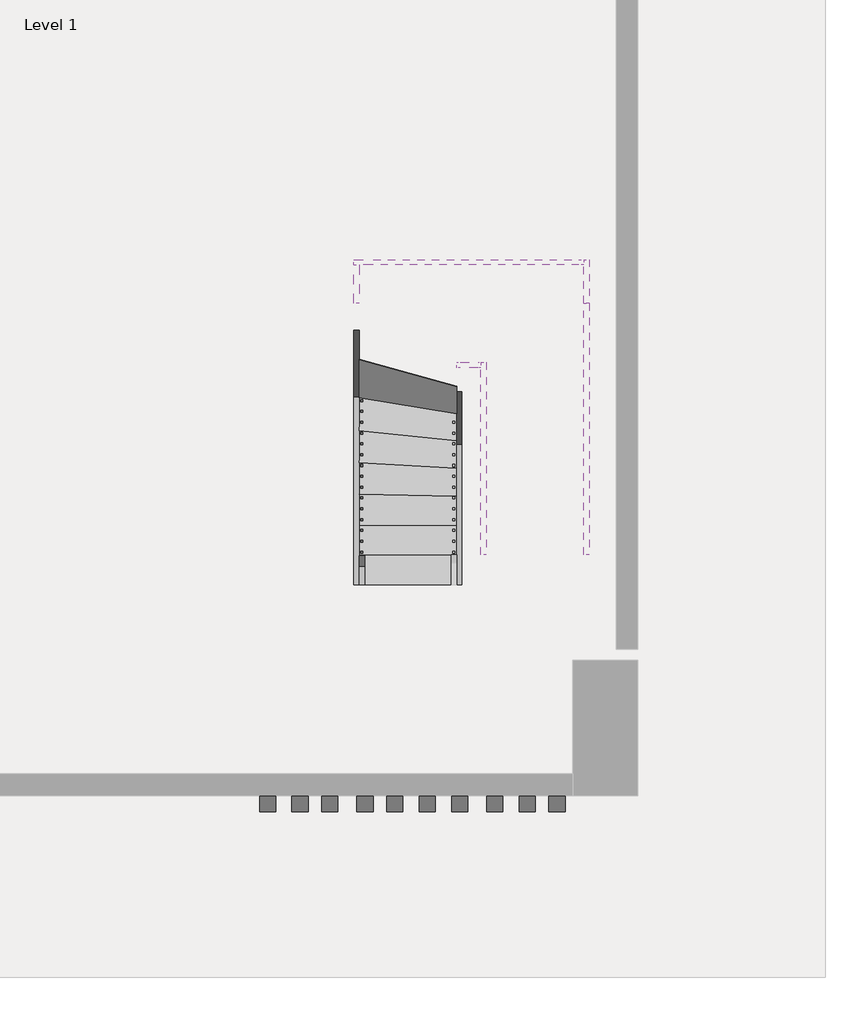
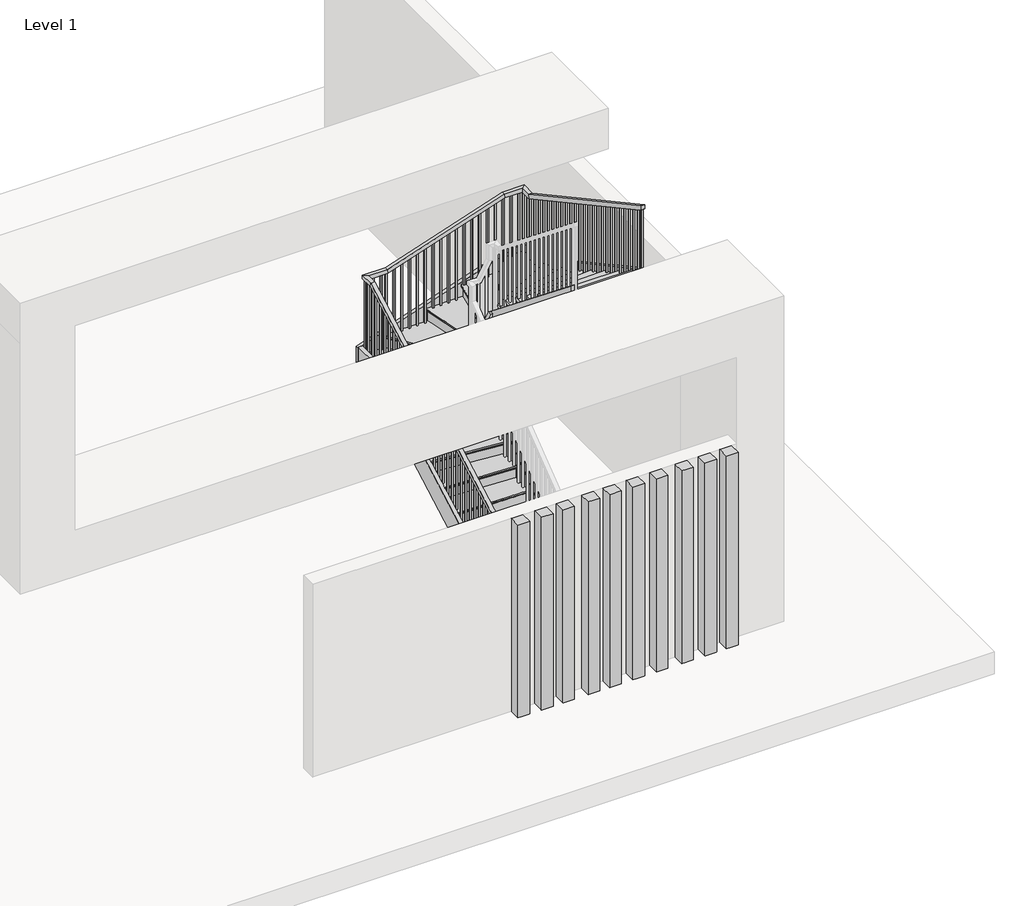
# One storey, part 2 of 2: 10 proxies, 8 members, 1 railing, 1 stair flight.
"""IFC4 building model written with IfcOpenShell, lengths in millimetres."""

from ifc_helpers import new_model, si_unit, frame, origin, origin_with_axes, place, context, project, spatial, polyline, outline, extrude, faceted_brep, transform, mapped, element, save
from components import stair_flight_b5c60846

model = new_model("IFC4")

# Units and contexts
model_context = context("Model", 3, world=origin())
ifc_project = project(units=[si_unit("LENGTHUNIT", "METRE", prefix="MILLI")], contexts=[model_context])

# Site, building, storey
site = spatial("IfcSite", under=ifc_project)
building = spatial("IfcBuilding", under=site)
storey = spatial("IfcBuildingStorey", under=building, Name="Level 1", Elevation=0.0)

# Proxies
placement = place(None, origin())
element("IfcBuildingElementProxy", 1, Name="Cornice", ObjectType="Cornice", at=placement, inside=storey, context=model_context, shape_type="SweptSolid", body=[
    extrude(outline(polyline([(-6255.4105967, 1286.2797066), (-6255.4105967, 1133.8797066), (-6407.8105967, 1133.8797066), (-6407.8105967, 1286.2797066), (-6255.4105967, 1286.2797066)])), origin_with_axes(), (0.0, 0.0, 1.0), 2659.145604),
])
element("IfcBuildingElementProxy", 2, Name="Cornice", ObjectType="Cornice", at=placement, inside=storey, context=model_context, shape_type="SweptSolid", body=[
    extrude(outline(polyline([(-5950.6105967, 1286.2797066), (-5950.6105967, 1133.8797066), (-6103.0105967, 1133.8797066), (-6103.0105967, 1286.2797066), (-5950.6105967, 1286.2797066)])), origin_with_axes(), (0.0, 0.0, 1.0), 2659.145604),
])
element("IfcBuildingElementProxy", 3, Name="Cornice", ObjectType="Cornice", at=placement, inside=storey, context=model_context, shape_type="SweptSolid", body=[
    extrude(outline(polyline([(-5671.2105967, 1286.2797066), (-5671.2105967, 1133.8797066), (-5823.6105967, 1133.8797066), (-5823.6105967, 1286.2797066), (-5671.2105967, 1286.2797066)])), origin_with_axes(), (0.0, 0.0, 1.0), 2659.145604),
])
element("IfcBuildingElementProxy", 4, Name="Cornice", ObjectType="Cornice", at=placement, inside=storey, context=model_context, shape_type="SweptSolid", body=[
    extrude(outline(polyline([(-5341.0105967, 1286.2797066), (-5341.0105967, 1133.8797066), (-5493.4105967, 1133.8797066), (-5493.4105967, 1286.2797066), (-5341.0105967, 1286.2797066)])), origin_with_axes(), (0.0, 0.0, 1.0), 2659.145604),
])
element("IfcBuildingElementProxy", 5, Name="Cornice", ObjectType="Cornice", at=placement, inside=storey, context=model_context, shape_type="SweptSolid", body=[
    extrude(outline(polyline([(-5061.6105967, 1286.2797066), (-5061.6105967, 1133.8797066), (-5214.0105967, 1133.8797066), (-5214.0105967, 1286.2797066), (-5061.6105967, 1286.2797066)])), origin_with_axes(), (0.0, 0.0, 1.0), 2659.145604),
])
element("IfcBuildingElementProxy", 6, Name="Cornice", ObjectType="Cornice", at=placement, inside=storey, context=model_context, shape_type="SweptSolid", body=[
    extrude(outline(polyline([(-4756.8105967, 1286.2797066), (-4756.8105967, 1133.8797066), (-4909.2105967, 1133.8797066), (-4909.2105967, 1286.2797066), (-4756.8105967, 1286.2797066)])), origin_with_axes(), (0.0, 0.0, 1.0), 2659.145604),
])
element("IfcBuildingElementProxy", 7, Name="Cornice", ObjectType="Cornice", at=placement, inside=storey, context=model_context, shape_type="SweptSolid", body=[
    extrude(outline(polyline([(-4452.0105967, 1286.2797066), (-4452.0105967, 1133.8797066), (-4604.4105967, 1133.8797066), (-4604.4105967, 1286.2797066), (-4452.0105967, 1286.2797066)])), origin_with_axes(), (0.0, 0.0, 1.0), 2659.145604),
])
element("IfcBuildingElementProxy", 8, Name="Cornice", ObjectType="Cornice", at=placement, inside=storey, context=model_context, shape_type="SweptSolid", body=[
    extrude(outline(polyline([(-4121.8105967, 1286.2797066), (-4121.8105967, 1133.8797066), (-4274.2105967, 1133.8797066), (-4274.2105967, 1286.2797066), (-4121.8105967, 1286.2797066)])), origin_with_axes(), (0.0, 0.0, 1.0), 2659.145604),
])
element("IfcBuildingElementProxy", 9, Name="Cornice", ObjectType="Cornice", at=placement, inside=storey, context=model_context, shape_type="SweptSolid", body=[
    extrude(outline(polyline([(-3817.0105967, 1286.2797066), (-3817.0105967, 1133.8797066), (-3969.4105967, 1133.8797066), (-3969.4105967, 1286.2797066), (-3817.0105967, 1286.2797066)])), origin_with_axes(), (0.0, 0.0, 1.0), 2659.145604),
])
element("IfcBuildingElementProxy", 10, Name="Cornice", ObjectType="Cornice", at=placement, inside=storey, context=model_context, shape_type="SweptSolid", body=[
    extrude(outline(polyline([(-3537.6105967, 1286.2797066), (-3537.6105967, 1133.8797066), (-3690.0105967, 1133.8797066), (-3690.0105967, 1286.2797066), (-3537.6105967, 1286.2797066)])), origin_with_axes(), (0.0, 0.0, 1.0), 2659.145604),
])

# Members
element("IfcMember", 11, ObjectType="Stringer - 2\" Width", at=placement, inside=storey, context=model_context, shape_type="SweptSolid", body=[
    extrude(outline(polyline([(3267.4797066, 0.0), (3267.4797066, 226.8967502), (5906.6355972, 1688.3473575), (5906.6355972, 1339.9346078), (3486.9189844, 0.0), (3267.4797066, 0.0)])), frame((-5523.3931367, 0.0, 0.0), z_axis=(1.0, 0.0, 0.0), x_axis=(0.0, 1.0, 0.0)), (0.0, 0.0, 1.0), 50.8),
])
element("IfcMember", 12, ObjectType="Stringer - 2\" Width", at=placement, inside=storey, context=model_context, shape_type="SweptSolid", body=[
    extrude(outline(polyline([(-5472.5931367, 5906.6355972), (-5523.3931367, 5906.6355972), (-5523.3931367, 6268.4113984), (-5472.5931367, 6268.4113984), (-5472.5931367, 5906.6355972)])), frame((0.0, 0.0, 1339.9346078), z_axis=(0.0, 0.0, 1.0), x_axis=(1.0, 0.0, 0.0)), (0.0, 0.0, 1.0), 348.4127497),
])
element("IfcMember", 13, ObjectType="Stringer - 2\" Width", at=placement, inside=storey, context=model_context, shape_type="SweptSolid", body=[
    extrude(outline(polyline([(1671.581207, -5523.3931367), (1383.5473575, -5523.3931367), (1383.5473575, -5340.4502408), (2035.7298543, -3364.3931367), (2369.5213068, -3364.3931367), (2369.5213068, -3408.6944146), (1671.581207, -5523.3931367)])), frame((0.0, 6268.4113984, 0.0), z_axis=(0.0, 1.0, 0.0), x_axis=(0.0, 0.0, 1.0)), (0.0, 0.0, 1.0), 50.8),
])
element("IfcMember", 14, ObjectType="Stringer - 2\" Width", at=placement, inside=storey, context=model_context, shape_type="SweptSolid", body=[
    extrude(outline(polyline([(-3364.3931367, 6319.2113984), (-3313.5931367, 6319.2113984), (-3313.5931367, 5909.577806), (-3364.3931367, 5909.577806), (-3364.3931367, 6319.2113984)])), frame((0.0, 0.0, 2048.5496929), z_axis=(0.0, 0.0, 1.0), x_axis=(1.0, 0.0, 0.0)), (0.0, 0.0, 1.0), 320.9716139),
])
element("IfcMember", 15, ObjectType="Stringer - 2\" Width", at=placement, inside=storey, context=model_context, shape_type="SweptSolid", body=[
    extrude(outline(polyline([(5909.577806, 2369.5213068), (5909.577806, 2048.5496929), (3546.8797066, 3333.0016037), (3546.8797066, 3653.9732176), (5909.577806, 2369.5213068)])), frame((-3364.3931367, 0.0, 0.0), z_axis=(1.0, 0.0, 0.0), x_axis=(0.0, 1.0, 0.0)), (0.0, 0.0, 1.0), 50.8),
])
element("IfcMember", 16, ObjectType="Stringer - 2\" Width", at=placement, inside=storey, context=model_context, shape_type="SweptSolid", body=[
    extrude(outline(polyline([(3267.4797066, 0.0), (3267.4797066, 188.0018686), (5303.2113984, 1759.6054409), (5303.2113984, 1374.5429999), (3522.7364772, 0.0), (3267.4797066, 0.0)])), frame((-4558.1931367, 0.0, 0.0), z_axis=(1.0, 0.0, 0.0), x_axis=(0.0, 1.0, 0.0)), (0.0, 0.0, 1.0), 50.8),
])
element("IfcMember", 17, ObjectType="Stringer - 2\" Width", at=placement, inside=storey, context=model_context, shape_type="SweptSolid", body=[
    extrude(outline(polyline([(1964.5655705, -4558.1931367), (1413.7610667, -4558.1931367), (1413.7610667, -4521.0415324), (1750.0370706, -4329.5931367), (2320.9680273, -4329.5931367), (2320.9680273, -4355.2863642), (1964.5655705, -4558.1931367)])), frame((0.0, 5303.2113984, 0.0), z_axis=(0.0, 1.0, 0.0), x_axis=(0.0, 0.0, 1.0)), (0.0, 0.0, 1.0), 50.8),
])
element("IfcMember", 18, ObjectType="Stringer - 2\" Width", at=placement, inside=storey, context=model_context, shape_type="SweptSolid", body=[
    extrude(outline(polyline([(5354.0113984, 2320.9680273), (5354.0113984, 1930.7796979), (3546.8797066, 3375.0977978), (3546.8797066, 3765.2861272), (5354.0113984, 2320.9680273)])), frame((-4329.5931367, 0.0, 0.0), z_axis=(1.0, 0.0, 0.0), x_axis=(0.0, 1.0, 0.0)), (0.0, 0.0, 1.0), 50.8),
])

# Railing
element("IfcRailing", 19, ObjectType="Handrail - Rectangular", at=placement, inside=storey, context=model_context, shape_type="SolidModel", body=[
    faceted_brep([(-5472.5931367, 3267.4797066, 1108.0231981), (-5472.5931367, 3267.4797066, 1049.9544064), (-5421.7931367, 3267.4797066, 1049.9544064), (-5421.7931367, 3267.4797066, 1108.0231981), (-5472.5931367, 6082.3927726, 2666.8005421), (-5472.5931367, 6095.5190966, 2616.0005421), (-5421.7931367, 6095.5190966, 2616.0005421), (-5421.7931367, 6082.3927726, 2666.8005421), (-5472.5931367, 6268.4113984, 2666.8005421), (-5472.5931367, 6268.4113984, 2616.0005421), (-5421.7931367, 6217.6113984, 2616.0005421), (-5421.7931367, 6217.6113984, 2666.8005421), (-5177.7014605, 6268.4113984, 2666.8005421), (-5169.5350263, 6268.4113984, 2616.0005421), (-5169.5350263, 6217.6113984, 2616.0005421), (-5177.7014605, 6217.6113984, 2666.8005421), (-3651.7050188, 6268.4113984, 3170.4439679), (-3643.5385846, 6268.4113984, 3119.6439679), (-3643.5385846, 6217.6113984, 3119.6439679), (-3651.7050188, 6217.6113984, 3170.4439679), (-3364.3931367, 6268.4113984, 3170.4439679), (-3364.3931367, 6268.4113984, 3119.6439679), (-3415.1931367, 6217.6113984, 3119.6439679), (-3415.1931367, 6217.6113984, 3170.4439679), (-3364.3931367, 6084.0047686, 3170.4439679), (-3364.3931367, 6071.0889723, 3119.6439679), (-3415.1931367, 6071.0889723, 3119.6439679), (-3415.1931367, 6084.0047686, 3170.4439679), (-3364.3931367, 3546.8797066, 4549.7209626), (-3415.1931367, 3546.8797066, 4549.7209626), (-3415.1931367, 3546.8797066, 4491.8994479), (-3364.3931367, 3546.8797066, 4491.8994479)], [[[0, 1, 2, 3]], [[1, 0, 4, 5]], [[2, 1, 5, 6]], [[3, 2, 6, 7]], [[0, 3, 7, 4]], [[5, 4, 8, 9]], [[6, 5, 9, 10]], [[7, 6, 10, 11]], [[4, 7, 11, 8]], [[9, 8, 12, 13]], [[10, 9, 13, 14]], [[11, 10, 14, 15]], [[8, 11, 15, 12]], [[13, 12, 16, 17]], [[14, 13, 17, 18]], [[15, 14, 18, 19]], [[12, 15, 19, 16]], [[17, 16, 20, 21]], [[18, 17, 21, 22]], [[19, 18, 22, 23]], [[16, 19, 23, 20]], [[21, 20, 24, 25]], [[22, 21, 25, 26]], [[23, 22, 26, 27]], [[20, 23, 27, 24]], [[28, 29, 30, 31]], [[25, 24, 28, 31]], [[26, 25, 31, 30]], [[27, 26, 30, 29]], [[24, 27, 29, 28]]]),
    extrude(outline(polyline([(3655.1297686, 4433.0506263), (3655.1297686, 3483.4285714), (3636.0797686, 3483.4285714), (3636.0797686, 4443.4069257), (3655.1297686, 4433.0506263)])), frame((-3399.3181367, 0.0, 0.0), z_axis=(1.0, 0.0, 0.0), x_axis=(0.0, 1.0, 0.0)), (0.0, 0.0, 1.0), 19.05),
    extrude(outline(polyline([(3756.7297686, 4377.8170295), (3756.7297686, 3483.4285714), (3737.6797686, 3483.4285714), (3737.6797686, 4388.1733289), (3756.7297686, 4377.8170295)])), frame((-3399.3181367, 0.0, 0.0), z_axis=(1.0, 0.0, 0.0), x_axis=(0.0, 1.0, 0.0)), (0.0, 0.0, 1.0), 19.05),
    extrude(outline(polyline([(3858.3297686, 4322.5834327), (3858.3297686, 3309.2571429), (3839.2797686, 3309.2571429), (3839.2797686, 4332.9397321), (3858.3297686, 4322.5834327)])), frame((-3399.3181367, 0.0, 0.0), z_axis=(1.0, 0.0, 0.0), x_axis=(0.0, 1.0, 0.0)), (0.0, 0.0, 1.0), 19.05),
    extrude(outline(polyline([(3959.9297686, 4267.349836), (3959.9297686, 3309.2571429), (3940.8797686, 3309.2571429), (3940.8797686, 4277.7061354), (3959.9297686, 4267.349836)])), frame((-3399.3181367, 0.0, 0.0), z_axis=(1.0, 0.0, 0.0), x_axis=(0.0, 1.0, 0.0)), (0.0, 0.0, 1.0), 19.05),
    extrude(outline(polyline([(4061.5297686, 4212.1162392), (4061.5297686, 3309.2571429), (4042.4797686, 3309.2571429), (4042.4797686, 4222.4725386), (4061.5297686, 4212.1162392)])), frame((-3399.3181367, 0.0, 0.0), z_axis=(1.0, 0.0, 0.0), x_axis=(0.0, 1.0, 0.0)), (0.0, 0.0, 1.0), 19.05),
    extrude(outline(polyline([(4163.1297686, 4156.8826424), (4163.1297686, 3135.0857143), (4144.0797686, 3135.0857143), (4144.0797686, 4167.2389418), (4163.1297686, 4156.8826424)])), frame((-3399.3181367, 0.0, 0.0), z_axis=(1.0, 0.0, 0.0), x_axis=(0.0, 1.0, 0.0)), (0.0, 0.0, 1.0), 19.05),
    extrude(outline(polyline([(4264.7297686, 4101.6490456), (4264.7297686, 3135.0857143), (4245.6797686, 3135.0857143), (4245.6797686, 4112.005345), (4264.7297686, 4101.6490456)])), frame((-3399.3181367, 0.0, 0.0), z_axis=(1.0, 0.0, 0.0), x_axis=(0.0, 1.0, 0.0)), (0.0, 0.0, 1.0), 19.05),
    extrude(outline(polyline([(4366.3297686, 4046.4154488), (4366.3297686, 3135.0857143), (4347.2797686, 3135.0857143), (4347.2797686, 4056.7717482), (4366.3297686, 4046.4154488)])), frame((-3399.3181367, 0.0, 0.0), z_axis=(1.0, 0.0, 0.0), x_axis=(0.0, 1.0, 0.0)), (0.0, 0.0, 1.0), 19.05),
    extrude(outline(polyline([(4467.9297686, 3991.1818521), (4467.9297686, 2960.9142857), (4448.8797686, 2960.9142857), (4448.8797686, 4001.5381515), (4467.9297686, 3991.1818521)])), frame((-3399.3181367, 0.0, 0.0), z_axis=(1.0, 0.0, 0.0), x_axis=(0.0, 1.0, 0.0)), (0.0, 0.0, 1.0), 19.05),
    extrude(outline(polyline([(4569.5297686, 3935.9482553), (4569.5297686, 2960.9142857), (4550.4797686, 2960.9142857), (4550.4797686, 3946.3045547), (4569.5297686, 3935.9482553)])), frame((-3399.3181367, 0.0, 0.0), z_axis=(1.0, 0.0, 0.0), x_axis=(0.0, 1.0, 0.0)), (0.0, 0.0, 1.0), 19.05),
    extrude(outline(polyline([(4671.1297686, 3880.7146585), (4671.1297686, 2960.9142857), (4652.0797686, 2960.9142857), (4652.0797686, 3891.0709579), (4671.1297686, 3880.7146585)])), frame((-3399.3181367, 0.0, 0.0), z_axis=(1.0, 0.0, 0.0), x_axis=(0.0, 1.0, 0.0)), (0.0, 0.0, 1.0), 19.05),
    extrude(outline(polyline([(4772.7297686, 3825.4810617), (4772.7297686, 2786.7428571), (4753.6797686, 2786.7428571), (4753.6797686, 3835.8373611), (4772.7297686, 3825.4810617)])), frame((-3399.3181367, 0.0, 0.0), z_axis=(1.0, 0.0, 0.0), x_axis=(0.0, 1.0, 0.0)), (0.0, 0.0, 1.0), 19.05),
    extrude(outline(polyline([(4874.3297686, 3770.2474649), (4874.3297686, 2786.7428571), (4855.2797686, 2786.7428571), (4855.2797686, 3780.6037643), (4874.3297686, 3770.2474649)])), frame((-3399.3181367, 0.0, 0.0), z_axis=(1.0, 0.0, 0.0), x_axis=(0.0, 1.0, 0.0)), (0.0, 0.0, 1.0), 19.05),
    extrude(outline(polyline([(4975.9297686, 3715.0138682), (4975.9297686, 2786.7428571), (4956.8797686, 2786.7428571), (4956.8797686, 3725.3701676), (4975.9297686, 3715.0138682)])), frame((-3399.3181367, 0.0, 0.0), z_axis=(1.0, 0.0, 0.0), x_axis=(0.0, 1.0, 0.0)), (0.0, 0.0, 1.0), 19.05),
    extrude(outline(polyline([(5077.5297686, 3659.7802714), (5077.5297686, 2612.5714286), (5058.4797686, 2612.5714286), (5058.4797686, 3670.1365708), (5077.5297686, 3659.7802714)])), frame((-3399.3181367, 0.0, 0.0), z_axis=(1.0, 0.0, 0.0), x_axis=(0.0, 1.0, 0.0)), (0.0, 0.0, 1.0), 19.05),
    extrude(outline(polyline([(5179.1297686, 3604.5466746), (5179.1297686, 2612.5714286), (5160.0797686, 2612.5714286), (5160.0797686, 3614.902974), (5179.1297686, 3604.5466746)])), frame((-3399.3181367, 0.0, 0.0), z_axis=(1.0, 0.0, 0.0), x_axis=(0.0, 1.0, 0.0)), (0.0, 0.0, 1.0), 19.05),
    extrude(outline(polyline([(5280.7297686, 3549.3130778), (5280.7297686, 2612.5714286), (5261.6797686, 2612.5714286), (5261.6797686, 3559.6693772), (5280.7297686, 3549.3130778)])), frame((-3399.3181367, 0.0, 0.0), z_axis=(1.0, 0.0, 0.0), x_axis=(0.0, 1.0, 0.0)), (0.0, 0.0, 1.0), 19.05),
    extrude(outline(polyline([(5382.3297686, 3494.0794811), (5382.3297686, 2438.4), (5363.2797686, 2438.4), (5363.2797686, 3504.4357804), (5382.3297686, 3494.0794811)])), frame((-3399.3181367, 0.0, 0.0), z_axis=(1.0, 0.0, 0.0), x_axis=(0.0, 1.0, 0.0)), (0.0, 0.0, 1.0), 19.05),
    extrude(outline(polyline([(5483.9297686, 3438.8458843), (5483.9297686, 2438.4), (5464.8797686, 2438.4), (5464.8797686, 3449.2021837), (5483.9297686, 3438.8458843)])), frame((-3399.3181367, 0.0, 0.0), z_axis=(1.0, 0.0, 0.0), x_axis=(0.0, 1.0, 0.0)), (0.0, 0.0, 1.0), 19.05),
    extrude(outline(polyline([(5585.5297686, 3383.6122875), (5585.5297686, 2438.4), (5566.4797686, 2438.4), (5566.4797686, 3393.9685869), (5585.5297686, 3383.6122875)])), frame((-3399.3181367, 0.0, 0.0), z_axis=(1.0, 0.0, 0.0), x_axis=(0.0, 1.0, 0.0)), (0.0, 0.0, 1.0), 19.05),
    extrude(outline(polyline([(5687.1297686, 3328.3786907), (5687.1297686, 2438.4), (5668.0797686, 2438.4), (5668.0797686, 3338.7349901), (5687.1297686, 3328.3786907)])), frame((-3399.3181367, 0.0, 0.0), z_axis=(1.0, 0.0, 0.0), x_axis=(0.0, 1.0, 0.0)), (0.0, 0.0, 1.0), 19.05),
    extrude(outline(polyline([(5788.7297686, 3273.1450939), (5788.7297686, 2264.2285714), (5769.6797686, 2264.2285714), (5769.6797686, 3283.5013933), (5788.7297686, 3273.1450939)])), frame((-3399.3181367, 0.0, 0.0), z_axis=(1.0, 0.0, 0.0), x_axis=(0.0, 1.0, 0.0)), (0.0, 0.0, 1.0), 19.05),
    extrude(outline(polyline([(5890.3297686, 3217.9114972), (5890.3297686, 2264.2285714), (5871.2797686, 2264.2285714), (5871.2797686, 3228.2677965), (5890.3297686, 3217.9114972)])), frame((-3399.3181367, 0.0, 0.0), z_axis=(1.0, 0.0, 0.0), x_axis=(0.0, 1.0, 0.0)), (0.0, 0.0, 1.0), 19.05),
    extrude(outline(polyline([(5991.9297686, 3162.6779004), (5991.9297686, 2264.2285714), (5972.8797686, 2264.2285714), (5972.8797686, 3173.0341998), (5991.9297686, 3162.6779004)])), frame((-3399.3181367, 0.0, 0.0), z_axis=(1.0, 0.0, 0.0), x_axis=(0.0, 1.0, 0.0)), (0.0, 0.0, 1.0), 19.05),
    extrude(outline(polyline([(-3380.2681367, 6150.9363984), (-3380.2681367, 6131.8863984), (-3399.3181367, 6131.8863984), (-3399.3181367, 6150.9363984), (-3380.2681367, 6150.9363984)])), frame((0.0, 0.0, 2264.2285714), z_axis=(0.0, 0.0, 1.0), x_axis=(1.0, 0.0, 0.0)), (0.0, 0.0, 1.0), 855.4153965),
    extrude(outline(polyline([(-3458.0300188, 6252.5363984), (-3438.9800188, 6252.5363984), (-3438.9800188, 6233.4863984), (-3458.0300188, 6233.4863984), (-3458.0300188, 6252.5363984)])), frame((0.0, 0.0, 2264.2285714), z_axis=(0.0, 0.0, 1.0), x_axis=(1.0, 0.0, 0.0)), (0.0, 0.0, 1.0), 855.4153965),
    extrude(outline(polyline([(-3559.6300188, 6252.5363984), (-3540.5800188, 6252.5363984), (-3540.5800188, 6233.4863984), (-3559.6300188, 6233.4863984), (-3559.6300188, 6252.5363984)])), frame((0.0, 0.0, 2264.2285714), z_axis=(0.0, 0.0, 1.0), x_axis=(1.0, 0.0, 0.0)), (0.0, 0.0, 1.0), 855.4153965),
    extrude(outline(polyline([(3113.1461354, -3663.2264605), (2090.0571429, -3663.2264605), (2090.0571429, -3644.1764605), (3119.4334419, -3644.1764605), (3113.1461354, -3663.2264605)])), frame((0.0, 6233.4863984, 0.0), z_axis=(0.0, 1.0, 0.0), x_axis=(0.0, 0.0, 1.0)), (0.0, 0.0, 1.0), 19.05),
    extrude(outline(polyline([(3079.6138344, -3764.8264605), (2090.0571429, -3764.8264605), (2090.0571429, -3745.7764605), (3085.9011408, -3745.7764605), (3079.6138344, -3764.8264605)])), frame((0.0, 6233.4863984, 0.0), z_axis=(0.0, 1.0, 0.0), x_axis=(0.0, 0.0, 1.0)), (0.0, 0.0, 1.0), 19.05),
    extrude(outline(polyline([(3046.0815334, -3866.4264605), (2090.0571429, -3866.4264605), (2090.0571429, -3847.3764605), (3052.3688398, -3847.3764605), (3046.0815334, -3866.4264605)])), frame((0.0, 6233.4863984, 0.0), z_axis=(0.0, 1.0, 0.0), x_axis=(0.0, 0.0, 1.0)), (0.0, 0.0, 1.0), 19.05),
    extrude(outline(polyline([(3012.5492323, -3968.0264605), (2090.0571429, -3968.0264605), (2090.0571429, -3948.9764605), (3018.8365388, -3948.9764605), (3012.5492323, -3968.0264605)])), frame((0.0, 6233.4863984, 0.0), z_axis=(0.0, 1.0, 0.0), x_axis=(0.0, 0.0, 1.0)), (0.0, 0.0, 1.0), 19.05),
    extrude(outline(polyline([(2979.0169313, -4069.6264605), (2090.0571429, -4069.6264605), (2090.0571429, -4050.5764605), (2985.3042377, -4050.5764605), (2979.0169313, -4069.6264605)])), frame((0.0, 6233.4863984, 0.0), z_axis=(0.0, 1.0, 0.0), x_axis=(0.0, 0.0, 1.0)), (0.0, 0.0, 1.0), 19.05),
    extrude(outline(polyline([(2945.4846303, -4171.2264605), (2090.0571429, -4171.2264605), (2090.0571429, -4152.1764605), (2951.7719367, -4152.1764605), (2945.4846303, -4171.2264605)])), frame((0.0, 6233.4863984, 0.0), z_axis=(0.0, 1.0, 0.0), x_axis=(0.0, 0.0, 1.0)), (0.0, 0.0, 1.0), 19.05),
    extrude(outline(polyline([(2911.9523292, -4272.8264605), (1915.8857143, -4272.8264605), (1915.8857143, -4253.7764605), (2918.2396357, -4253.7764605), (2911.9523292, -4272.8264605)])), frame((0.0, 6233.4863984, 0.0), z_axis=(0.0, 1.0, 0.0), x_axis=(0.0, 0.0, 1.0)), (0.0, 0.0, 1.0), 19.05),
    extrude(outline(polyline([(2878.4200282, -4374.4264605), (1915.8857143, -4374.4264605), (1915.8857143, -4355.3764605), (2884.7073346, -4355.3764605), (2878.4200282, -4374.4264605)])), frame((0.0, 6233.4863984, 0.0), z_axis=(0.0, 1.0, 0.0), x_axis=(0.0, 0.0, 1.0)), (0.0, 0.0, 1.0), 19.05),
    extrude(outline(polyline([(2844.8877272, -4476.0264605), (1915.8857143, -4476.0264605), (1915.8857143, -4456.9764605), (2851.1750336, -4456.9764605), (2844.8877272, -4476.0264605)])), frame((0.0, 6233.4863984, 0.0), z_axis=(0.0, 1.0, 0.0), x_axis=(0.0, 0.0, 1.0)), (0.0, 0.0, 1.0), 19.05),
    extrude(outline(polyline([(2811.3554261, -4577.6264605), (1915.8857143, -4577.6264605), (1915.8857143, -4558.5764605), (2817.6427326, -4558.5764605), (2811.3554261, -4577.6264605)])), frame((0.0, 6233.4863984, 0.0), z_axis=(0.0, 1.0, 0.0), x_axis=(0.0, 0.0, 1.0)), (0.0, 0.0, 1.0), 19.05),
    extrude(outline(polyline([(2777.8231251, -4679.2264605), (1741.7142857, -4679.2264605), (1741.7142857, -4660.1764605), (2784.1104315, -4660.1764605), (2777.8231251, -4679.2264605)])), frame((0.0, 6233.4863984, 0.0), z_axis=(0.0, 1.0, 0.0), x_axis=(0.0, 0.0, 1.0)), (0.0, 0.0, 1.0), 19.05),
    extrude(outline(polyline([(2744.2908241, -4780.8264605), (1741.7142857, -4780.8264605), (1741.7142857, -4761.7764605), (2750.5781305, -4761.7764605), (2744.2908241, -4780.8264605)])), frame((0.0, 6233.4863984, 0.0), z_axis=(0.0, 1.0, 0.0), x_axis=(0.0, 0.0, 1.0)), (0.0, 0.0, 1.0), 19.05),
    extrude(outline(polyline([(2710.758523, -4882.4264605), (1741.7142857, -4882.4264605), (1741.7142857, -4863.3764605), (2717.0458295, -4863.3764605), (2710.758523, -4882.4264605)])), frame((0.0, 6233.4863984, 0.0), z_axis=(0.0, 1.0, 0.0), x_axis=(0.0, 0.0, 1.0)), (0.0, 0.0, 1.0), 19.05),
    extrude(outline(polyline([(2677.226222, -4984.0264605), (1741.7142857, -4984.0264605), (1741.7142857, -4964.9764605), (2683.5135284, -4964.9764605), (2677.226222, -4984.0264605)])), frame((0.0, 6233.4863984, 0.0), z_axis=(0.0, 1.0, 0.0), x_axis=(0.0, 0.0, 1.0)), (0.0, 0.0, 1.0), 19.05),
    extrude(outline(polyline([(2643.693921, -5085.6264605), (1741.7142857, -5085.6264605), (1741.7142857, -5066.5764605), (2649.9812274, -5066.5764605), (2643.693921, -5085.6264605)])), frame((0.0, 6233.4863984, 0.0), z_axis=(0.0, 1.0, 0.0), x_axis=(0.0, 0.0, 1.0)), (0.0, 0.0, 1.0), 19.05),
    extrude(outline(polyline([(-5253.5181367, 6252.5363984), (-5234.4681367, 6252.5363984), (-5234.4681367, 6233.4863984), (-5253.5181367, 6233.4863984), (-5253.5181367, 6252.5363984)])), frame((0.0, 0.0, 1567.5428571), z_axis=(0.0, 0.0, 1.0), x_axis=(1.0, 0.0, 0.0)), (0.0, 0.0, 1.0), 1048.457685),
    extrude(outline(polyline([(-5355.1181367, 6252.5363984), (-5336.0681367, 6252.5363984), (-5336.0681367, 6233.4863984), (-5355.1181367, 6233.4863984), (-5355.1181367, 6252.5363984)])), frame((0.0, 0.0, 1567.5428571), z_axis=(0.0, 0.0, 1.0), x_axis=(1.0, 0.0, 0.0)), (0.0, 0.0, 1.0), 1048.457685),
    extrude(outline(polyline([(-5456.7181367, 6174.4677726), (-5456.7181367, 6193.5177726), (-5437.6681367, 6193.5177726), (-5437.6681367, 6174.4677726), (-5456.7181367, 6174.4677726)])), frame((0.0, 0.0, 1567.5428571), z_axis=(0.0, 0.0, 1.0), x_axis=(1.0, 0.0, 0.0)), (0.0, 0.0, 1.0), 1048.457685),
    extrude(outline(polyline([(6020.2047066, 2574.294684), (6020.2047066, 1567.5428571), (6001.1547066, 1567.5428571), (6001.1547066, 2563.7456164), (6020.2047066, 2574.294684)])), frame((-5456.7181367, 0.0, 0.0), z_axis=(1.0, 0.0, 0.0), x_axis=(0.0, 1.0, 0.0)), (0.0, 0.0, 1.0), 19.05),
    extrude(outline(polyline([(5918.6047066, 2518.0329898), (5918.6047066, 1567.5428571), (5899.5547066, 1567.5428571), (5899.5547066, 2507.4839222), (5918.6047066, 2518.0329898)])), frame((-5456.7181367, 0.0, 0.0), z_axis=(1.0, 0.0, 0.0), x_axis=(0.0, 1.0, 0.0)), (0.0, 0.0, 1.0), 19.05),
    extrude(outline(polyline([(5817.0047066, 2461.7712956), (5817.0047066, 1567.5428571), (5797.9547066, 1567.5428571), (5797.9547066, 2451.222228), (5817.0047066, 2461.7712956)])), frame((-5456.7181367, 0.0, 0.0), z_axis=(1.0, 0.0, 0.0), x_axis=(0.0, 1.0, 0.0)), (0.0, 0.0, 1.0), 19.05),
    extrude(outline(polyline([(5715.4047066, 2405.5096014), (5715.4047066, 1393.3714286), (5696.3547066, 1393.3714286), (5696.3547066, 2394.9605337), (5715.4047066, 2405.5096014)])), frame((-5456.7181367, 0.0, 0.0), z_axis=(1.0, 0.0, 0.0), x_axis=(0.0, 1.0, 0.0)), (0.0, 0.0, 1.0), 19.05),
    extrude(outline(polyline([(5613.8047066, 2349.2479072), (5613.8047066, 1393.3714286), (5594.7547066, 1393.3714286), (5594.7547066, 2338.6988395), (5613.8047066, 2349.2479072)])), frame((-5456.7181367, 0.0, 0.0), z_axis=(1.0, 0.0, 0.0), x_axis=(0.0, 1.0, 0.0)), (0.0, 0.0, 1.0), 19.05),
    extrude(outline(polyline([(5512.2047066, 2292.986213), (5512.2047066, 1393.3714286), (5493.1547066, 1393.3714286), (5493.1547066, 2282.4371453), (5512.2047066, 2292.986213)])), frame((-5456.7181367, 0.0, 0.0), z_axis=(1.0, 0.0, 0.0), x_axis=(0.0, 1.0, 0.0)), (0.0, 0.0, 1.0), 19.05),
    extrude(outline(polyline([(5410.6047066, 2236.7245188), (5410.6047066, 1393.3714286), (5391.5547066, 1393.3714286), (5391.5547066, 2226.1754511), (5410.6047066, 2236.7245188)])), frame((-5456.7181367, 0.0, 0.0), z_axis=(1.0, 0.0, 0.0), x_axis=(0.0, 1.0, 0.0)), (0.0, 0.0, 1.0), 19.05),
    extrude(outline(polyline([(5309.0047066, 2180.4628245), (5309.0047066, 1219.2), (5289.9547066, 1219.2), (5289.9547066, 2169.9137569), (5309.0047066, 2180.4628245)])), frame((-5456.7181367, 0.0, 0.0), z_axis=(1.0, 0.0, 0.0), x_axis=(0.0, 1.0, 0.0)), (0.0, 0.0, 1.0), 19.05),
    extrude(outline(polyline([(5207.4047066, 2124.2011303), (5207.4047066, 1219.2), (5188.3547066, 1219.2), (5188.3547066, 2113.6520627), (5207.4047066, 2124.2011303)])), frame((-5456.7181367, 0.0, 0.0), z_axis=(1.0, 0.0, 0.0), x_axis=(0.0, 1.0, 0.0)), (0.0, 0.0, 1.0), 19.05),
    extrude(outline(polyline([(5105.8047066, 2067.9394361), (5105.8047066, 1219.2), (5086.7547066, 1219.2), (5086.7547066, 2057.3903685), (5105.8047066, 2067.9394361)])), frame((-5456.7181367, 0.0, 0.0), z_axis=(1.0, 0.0, 0.0), x_axis=(0.0, 1.0, 0.0)), (0.0, 0.0, 1.0), 19.05),
    extrude(outline(polyline([(5004.2047066, 2011.6777419), (5004.2047066, 1045.0285714), (4985.1547066, 1045.0285714), (4985.1547066, 2001.1286742), (5004.2047066, 2011.6777419)])), frame((-5456.7181367, 0.0, 0.0), z_axis=(1.0, 0.0, 0.0), x_axis=(0.0, 1.0, 0.0)), (0.0, 0.0, 1.0), 19.05),
    extrude(outline(polyline([(4902.6047066, 1955.4160477), (4902.6047066, 1045.0285714), (4883.5547066, 1045.0285714), (4883.5547066, 1944.86698), (4902.6047066, 1955.4160477)])), frame((-5456.7181367, 0.0, 0.0), z_axis=(1.0, 0.0, 0.0), x_axis=(0.0, 1.0, 0.0)), (0.0, 0.0, 1.0), 19.05),
    extrude(outline(polyline([(4801.0047066, 1899.1543535), (4801.0047066, 1045.0285714), (4781.9547066, 1045.0285714), (4781.9547066, 1888.6052858), (4801.0047066, 1899.1543535)])), frame((-5456.7181367, 0.0, 0.0), z_axis=(1.0, 0.0, 0.0), x_axis=(0.0, 1.0, 0.0)), (0.0, 0.0, 1.0), 19.05),
    extrude(outline(polyline([(4699.4047066, 1842.8926593), (4699.4047066, 870.8571429), (4680.3547066, 870.8571429), (4680.3547066, 1832.3435916), (4699.4047066, 1842.8926593)])), frame((-5456.7181367, 0.0, 0.0), z_axis=(1.0, 0.0, 0.0), x_axis=(0.0, 1.0, 0.0)), (0.0, 0.0, 1.0), 19.05),
    extrude(outline(polyline([(4597.8047066, 1786.6309651), (4597.8047066, 870.8571429), (4578.7547066, 870.8571429), (4578.7547066, 1776.0818974), (4597.8047066, 1786.6309651)])), frame((-5456.7181367, 0.0, 0.0), z_axis=(1.0, 0.0, 0.0), x_axis=(0.0, 1.0, 0.0)), (0.0, 0.0, 1.0), 19.05),
    extrude(outline(polyline([(4496.2047066, 1730.3692708), (4496.2047066, 870.8571429), (4477.1547066, 870.8571429), (4477.1547066, 1719.8202032), (4496.2047066, 1730.3692708)])), frame((-5456.7181367, 0.0, 0.0), z_axis=(1.0, 0.0, 0.0), x_axis=(0.0, 1.0, 0.0)), (0.0, 0.0, 1.0), 19.05),
    extrude(outline(polyline([(4394.6047066, 1674.1075766), (4394.6047066, 696.6857143), (4375.5547066, 696.6857143), (4375.5547066, 1663.558509), (4394.6047066, 1674.1075766)])), frame((-5456.7181367, 0.0, 0.0), z_axis=(1.0, 0.0, 0.0), x_axis=(0.0, 1.0, 0.0)), (0.0, 0.0, 1.0), 19.05),
    extrude(outline(polyline([(4293.0047066, 1617.8458824), (4293.0047066, 696.6857143), (4273.9547066, 696.6857143), (4273.9547066, 1607.2968147), (4293.0047066, 1617.8458824)])), frame((-5456.7181367, 0.0, 0.0), z_axis=(1.0, 0.0, 0.0), x_axis=(0.0, 1.0, 0.0)), (0.0, 0.0, 1.0), 19.05),
    extrude(outline(polyline([(4191.4047066, 1561.5841882), (4191.4047066, 696.6857143), (4172.3547066, 696.6857143), (4172.3547066, 1551.0351205), (4191.4047066, 1561.5841882)])), frame((-5456.7181367, 0.0, 0.0), z_axis=(1.0, 0.0, 0.0), x_axis=(0.0, 1.0, 0.0)), (0.0, 0.0, 1.0), 19.05),
    extrude(outline(polyline([(4089.8047066, 1505.322494), (4089.8047066, 522.5142857), (4070.7547066, 522.5142857), (4070.7547066, 1494.7734263), (4089.8047066, 1505.322494)])), frame((-5456.7181367, 0.0, 0.0), z_axis=(1.0, 0.0, 0.0), x_axis=(0.0, 1.0, 0.0)), (0.0, 0.0, 1.0), 19.05),
    extrude(outline(polyline([(3988.2047066, 1449.0607998), (3988.2047066, 522.5142857), (3969.1547066, 522.5142857), (3969.1547066, 1438.5117321), (3988.2047066, 1449.0607998)])), frame((-5456.7181367, 0.0, 0.0), z_axis=(1.0, 0.0, 0.0), x_axis=(0.0, 1.0, 0.0)), (0.0, 0.0, 1.0), 19.05),
    extrude(outline(polyline([(3886.6047066, 1392.7991056), (3886.6047066, 522.5142857), (3867.5547066, 522.5142857), (3867.5547066, 1382.2500379), (3886.6047066, 1392.7991056)])), frame((-5456.7181367, 0.0, 0.0), z_axis=(1.0, 0.0, 0.0), x_axis=(0.0, 1.0, 0.0)), (0.0, 0.0, 1.0), 19.05),
    extrude(outline(polyline([(3785.0047066, 1336.5374113), (3785.0047066, 348.3428571), (3765.9547066, 348.3428571), (3765.9547066, 1325.9883437), (3785.0047066, 1336.5374113)])), frame((-5456.7181367, 0.0, 0.0), z_axis=(1.0, 0.0, 0.0), x_axis=(0.0, 1.0, 0.0)), (0.0, 0.0, 1.0), 19.05),
    extrude(outline(polyline([(3683.4047066, 1280.2757171), (3683.4047066, 348.3428571), (3664.3547066, 348.3428571), (3664.3547066, 1269.7266495), (3683.4047066, 1280.2757171)])), frame((-5456.7181367, 0.0, 0.0), z_axis=(1.0, 0.0, 0.0), x_axis=(0.0, 1.0, 0.0)), (0.0, 0.0, 1.0), 19.05),
    extrude(outline(polyline([(3581.8047066, 1224.0140229), (3581.8047066, 348.3428571), (3562.7547066, 348.3428571), (3562.7547066, 1213.4649553), (3581.8047066, 1224.0140229)])), frame((-5456.7181367, 0.0, 0.0), z_axis=(1.0, 0.0, 0.0), x_axis=(0.0, 1.0, 0.0)), (0.0, 0.0, 1.0), 19.05),
    extrude(outline(polyline([(3480.2047066, 1167.7523287), (3480.2047066, 174.1714286), (3461.1547066, 174.1714286), (3461.1547066, 1157.203261), (3480.2047066, 1167.7523287)])), frame((-5456.7181367, 0.0, 0.0), z_axis=(1.0, 0.0, 0.0), x_axis=(0.0, 1.0, 0.0)), (0.0, 0.0, 1.0), 19.05),
    extrude(outline(polyline([(3378.6047066, 1111.4906345), (3378.6047066, 174.1714286), (3359.5547066, 174.1714286), (3359.5547066, 1100.9415668), (3378.6047066, 1111.4906345)])), frame((-5456.7181367, 0.0, 0.0), z_axis=(1.0, 0.0, 0.0), x_axis=(0.0, 1.0, 0.0)), (0.0, 0.0, 1.0), 19.05),
    extrude(outline(polyline([(-3380.2681367, 6093.5297686), (-3380.2681367, 6074.4797686), (-3399.3181367, 6074.4797686), (-3399.3181367, 6093.5297686), (-3380.2681367, 6093.5297686)])), frame((0.0, 0.0, 2264.2285714), z_axis=(0.0, 0.0, 1.0), x_axis=(1.0, 0.0, 0.0)), (0.0, 0.0, 1.0), 855.4153965),
    extrude(outline(polyline([(-3399.3181367, 6252.5363984), (-3380.2681367, 6252.5363984), (-3380.2681367, 6233.4863984), (-3399.3181367, 6233.4863984), (-3399.3181367, 6252.5363984)])), frame((0.0, 0.0, 2264.2285714), z_axis=(0.0, 0.0, 1.0), x_axis=(1.0, 0.0, 0.0)), (0.0, 0.0, 1.0), 855.4153965),
    extrude(outline(polyline([(3113.8050457, -3661.2300188), (2090.0571429, -3661.2300188), (2090.0571429, -3642.1800188), (3120.0923522, -3642.1800188), (3113.8050457, -3661.2300188)])), frame((0.0, 6233.4863984, 0.0), z_axis=(0.0, 1.0, 0.0), x_axis=(0.0, 0.0, 1.0)), (0.0, 0.0, 1.0), 19.05),
    extrude(outline(polyline([(-5187.2264605, 6252.5363984), (-5168.1764605, 6252.5363984), (-5168.1764605, 6233.4863984), (-5187.2264605, 6233.4863984), (-5187.2264605, 6252.5363984)])), frame((0.0, 0.0, 1741.7142857), z_axis=(0.0, 0.0, 1.0), x_axis=(1.0, 0.0, 0.0)), (0.0, 0.0, 1.0), 874.2862564),
    extrude(outline(polyline([(-5456.7181367, 6233.4863984), (-5456.7181367, 6252.5363984), (-5437.6681367, 6252.5363984), (-5437.6681367, 6233.4863984), (-5456.7181367, 6233.4863984)])), frame((0.0, 0.0, 1567.5428571), z_axis=(0.0, 0.0, 1.0), x_axis=(1.0, 0.0, 0.0)), (0.0, 0.0, 1.0), 1048.457685),
    extrude(outline(polyline([(6091.9177726, 2614.0062844), (6091.9177726, 1567.5428571), (6072.8677726, 1567.5428571), (6072.8677726, 2603.4572167), (6091.9177726, 2614.0062844)])), frame((-5456.7181367, 0.0, 0.0), z_axis=(1.0, 0.0, 0.0), x_axis=(0.0, 1.0, 0.0)), (0.0, 0.0, 1.0), 19.05),
    extrude(outline(polyline([(3565.9297066, 4481.5431486), (3565.9297066, 3483.4285714), (3546.8797066, 3483.4285714), (3546.8797066, 4491.8994479), (3565.9297066, 4481.5431486)])), frame((-3399.3181367, 0.0, 0.0), z_axis=(1.0, 0.0, 0.0), x_axis=(0.0, 1.0, 0.0)), (0.0, 0.0, 1.0), 19.05),
    extrude(outline(polyline([(3286.5297066, 1060.5034741), (3286.5297066, 174.1714286), (3267.4797066, 174.1714286), (3267.4797066, 1049.9544064), (3286.5297066, 1060.5034741)])), frame((-5456.7181367, 0.0, 0.0), z_axis=(1.0, 0.0, 0.0), x_axis=(0.0, 1.0, 0.0)), (0.0, 0.0, 1.0), 19.05),
])

# Stair flight
stair_flight_shape = stair_flight_b5c60846(model_context)
element("IfcStairFlight", 20, ObjectType="2\" Tread 1\" Nosing 1/4\" Riser", at=placement, inside=storey, context=model_context, shape_type="MappedRepresentation", body=[
    mapped(stair_flight_shape, transform((0.0, 0.0, 0.0), x_axis=(1.0, 0.0, 0.0), y_axis=(0.0, 1.0, 0.0), z_axis=(0.0, 0.0, 1.0))),
])

save(model, "model.ifc")

# Revit data of these elements
# Type "Handrail - Rectangular"
#   Assembly Code = "C2010400"
#   built-in parameter 1008612 = 0.0416667 (stored number, unit not read)
#   built-in parameter 1008611 = 0.0416667 (stored number, unit not read)
#   built-in parameter 1008609 = 0.333333 (stored number, unit not read)
#   built-in parameter 1008604 = 0.166667 (stored number, unit not read)
#   built-in parameter 1008603 = 0.166667 (stored number, unit not read)
#   Railing Height = 3' - 0"
#   built-in parameter 1008630 = 2
#   built-in parameter 1008610 = 2
#   built-in parameter 1008618 = Baluster - Square : 3/4"
# Elements 1, 2, 3, 4, 5, 6, 7, 8, 9, 10 (IfcBuildingElementProxy, "Cornice")
#   Phase Created = New Construction
#   Materials on its faces: "Default Wall"
# Elements 11, 12, 13, 14, 15, 16, 17, 18 (IfcMember, "Stringer - 2\" Width")
#   Phase Created = New Construction
# Element 19 (IfcRailing, "Handrail - Rectangular")
#   Phase Created = New Construction
# Element 20 (IfcStairFlight, "2\" Tread 1\" Nosing 1/4\" Riser")
#   Phase Created = New Construction
# Materials
#   "Default Wall": colour RGB 128 128 128, transparency 0
